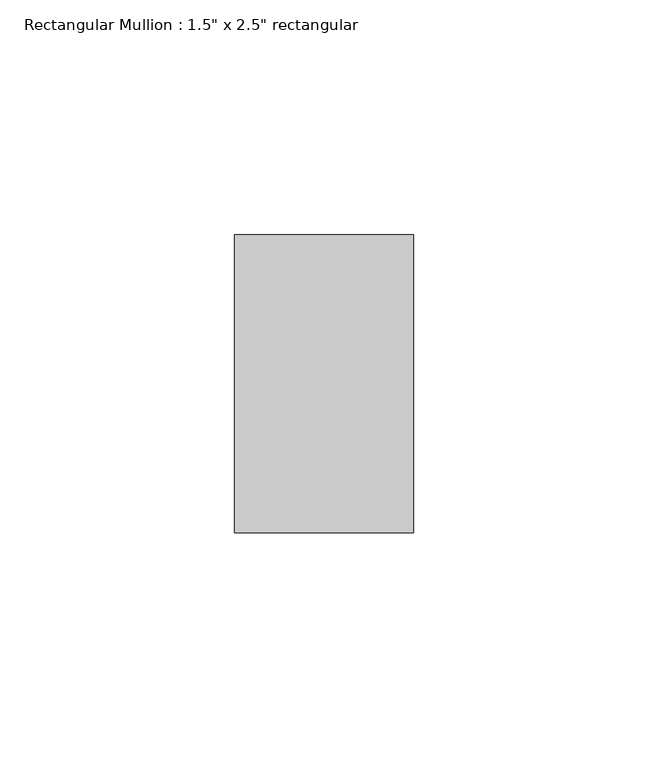
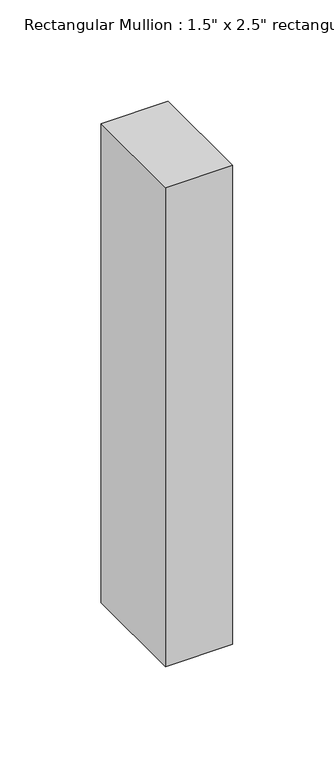
"""IFC4 building model written with IfcOpenShell, lengths in millimetres: member geometry."""

from ifc_helpers import new_model, si_unit, frame, origin, place, context, project, spatial, polyline, outline, extrude, source, transform, mapped, element, save


def member_06854975(model_context):
    return source(origin(), model_context, "Body", "SweptSolid", [
        extrude(outline(polyline([(0.0, 31.75), (0.0, -31.75), (-38.1, -31.75), (-38.1, 31.75), (0.0, 31.75)])), frame((0.0, 0.0, -288.2320668), z_axis=(0.0, 0.0, 1.0), x_axis=(1.0, 0.0, 0.0)), (0.0, 0.0, 1.0), 288.2320668),
    ])


if __name__ == "__main__":
    model = new_model("IFC4")
    model_context = context("Model", 3, world=origin())
    ifc_project = project(units=[si_unit("LENGTHUNIT", "METRE", prefix="MILLI")], contexts=[model_context])
    site = spatial("IfcSite", under=ifc_project)
    building = spatial("IfcBuilding", under=site)
    placement = place(None, origin())
    member_shape = member_06854975(model_context)
    element("IfcMember", 1, ObjectType="Rectangular Mullion : 1.5\" x 2.5\" rectangular", at=placement, inside=building, context=model_context, shape_type="MappedRepresentation", body=[
        mapped(member_shape, transform((0.0, 0.0, 0.0), x_axis=(1.0, 0.0, 0.0), y_axis=(0.0, 1.0, 0.0), z_axis=(0.0, 0.0, 1.0))),
    ])
    save(model, "model.ifc")

# Revit data of these elements
# Type "Rectangular Mullion : 1.5\" x 2.5\" rectangular"
#   built-in parameter 1007304 = 0.208333 (stored number, unit not read)
#   built-in parameter 1007301 = 0.0625 (stored number, unit not read)
#   built-in parameter 1007300 = 0.0625 (stored number, unit not read)
# Element 1 (IfcMember, "Rectangular Mullion : 1.5\" x 2.5\" rectangular")
#   Materials on its faces: "Aluminum"
# Materials
#   "Aluminum": class "Metal", colour RGB 247 247 247, transparency 0, Description = "Aluminum 6061", Cost = 0
